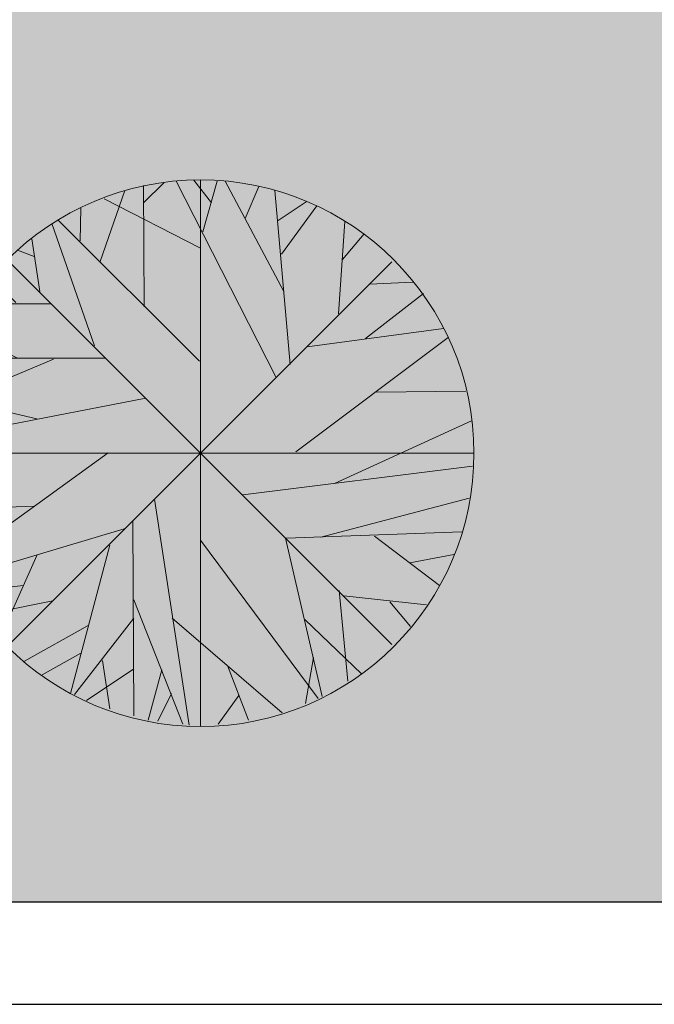
# Model space of a CAD drawing. Units: inches. Extents: x 459864 to 460310, y 324185 to 324787.
# Tile 72 of 112: x 460210 to 460238, y 324195 to 324238. Entities that reach past the tile are written whole.
import ezdxf

# ---------------------------------------------------------------- set-up
doc = ezdxf.new("R2010")
doc.units = ezdxf.units.IN
for name, color, linetype, lineweight in [('C-PROP', 7, 'Continuous', 30), ('L-PLNT', 3, 'Continuous', 13), ('L-SITE-PATT', 252, 'Continuous', 13)]:
    doc.layers.add(name, color=color, linetype=linetype, lineweight=lineweight)

# ---------------------------------------------------------------- blocks, each defined once
blk = doc.blocks.new('Tree - deciduous plan')
for p, q in [((-12.5388, 54.9406), (-7.9613, 59.4546)), ((-12.3627, 32.1443), (-12.5388, 58.7776)), ((-5.3205, 59.6806), (16.5105, 16.7963)), ((2.426, 54.9406), (-1.4472, 59.9056)), ((0, 59.9996), (0, -60)), ((0.4894, 48.6208), (3.6584, 59.6806)), ((18.2711, 35.5298), (5.419, 59.6806)), ((9.8203, 51.5549), (12.8133, 58.5516)), ((-22.0458, 42.0753), (-16.5881, 57.6486)), ((19.6795, 19.5047), (16.3344, 57.6486)), ((-21.1656, 55.8436), (-0.0388, 45.0094)), ((17.0387, 51.1035), (23.2006, 55.1666)), ((17.7429, 43.6552), (25.4894, 54.2636)), ((-26.4472, 46.5894), (-26.2712, 53.8116)), ((-32.6092, 50.4264), (-23.2782, 23.5674)), ((-31.2008, 51.1035), (-0.2149, 20.1818)), ((31.6513, 50.8778), (30.2429, 30.5643)), ((31.1232, 42.5267), (35.8767, 48.1693)), ((-37.0107, 47.0408), (-35.25, 35.5298)), ((-40.1797, 44.558), (-36.4825, 43.2038)), ((42, 42), (-42, -42)), ((42, -42), (-42, 42)), ((-43.8768, 36.4326), (-44.405, 40.2696)), ((-45.8134, 38.2383), (-40.5318, 33.0471)), ((37.1091, 37.1098), (46.6161, 37.5612)), ((36.2288, 25.1474), (48.9049, 35.0784)), ((-49.8627, 32.8214), (-32.7853, 32.8214)), ((-53.2078, 27.4044), (-40.1797, 20.859)), ((23.3767, 23.3417), (53.3063, 27.4044)), ((-54.7923, 24.4702), (-47.75, 21.0847)), ((54.3626, 25.3731), (20.9119, 0.3198)), ((-32.2571, 20.6333), (-59.1937, 9.348)), ((-56.0247, 20.859), (-20.8134, 20.859)), ((-57.081, 17.9248), (-47.0458, 14.7649)), ((38.5175, 13.4107), (58.2359, 13.6364)), ((-59.7219, 2.8025), (-12.0106, 12.0565)), ((-58.6656, 12.7336), (-35.9543, 7.5424)), ((29.3626, -6.6771), (59.4682, 7.091)), ((-54.6162, -24.7335), (-20.2853, 0.0941)), ((-60, 0), (60, 0)), ((-45.2853, -0.1316), (-59.0177, -10.0627)), ((9.2922, -9.1598), (59.6443, -2.8401)), ((-59.7219, -4.8714), (-54.2641, -6.6771)), ((-10.074, -10.0627), (-2.5036, -59.7178)), ((26.3697, -18.4138), (58.9401, -9.8369)), ((-58.4895, -12.3197), (-36.4825, -11.6426)), ((-14.8275, -15.0282), (-14.6515, -57.6865)), ((-53.2078, -27.442), (-16.7641, -16.6081)), ((18.7992, -18.6394), (57.3556, -17.2853)), ((-57.081, -18.4138), (-45.2853, -17.9624)), ((-52.6797, -18.188), (-55.4966, -22.0251)), ((-47.2219, -19.3166), (-50.2148, -26.3135)), ((-0.0388, -19.0909), (25.8415, -53.8495)), ((18.6232, -18.6394), (26.7218, -53.3981)), ((38.1654, -18.188), (52.426, -29.0219)), ((-19.9331, -20.2194), (-28.5599, -52.721)), ((-35.9543, -22.4765), (-44.0529, -40.5329)), ((45.9119, -24.0564), (55.595, -22.2508)), ((-38.9472, -29.0219), (-51.4472, -30.6018)), ((-46.5177, -30.1504), (-49.5106, -33.536)), ((30.419, -30.1504), (32.3556, -50.0125)), ((-32.4331, -32.4075), (-48.1021, -35.5674)), ((-14.6515, -32.1818), (-3.912, -59.4922)), ((31.4753, -31.279), (49.6091, -33.3103)), ((41.5105, -32.6332), (46.088, -38.0501)), ((-43.7008, -34.6645), (-46.6937, -37.373)), ((-14.6515, -36.2445), (-27.6797, -52.9467)), ((-6.2008, -36.2445), (17.919, -57.0094)), ((22.8485, -36.4702), (35.3485, -48.4326)), ((-24.6867, -37.8244), (-38.7712, -45.7241)), ((-26.2712, -43.9185), (-34.7219, -48.6583)), ((24.7852, -44.8213), (23.0246, -54.978)), ((-14.6515, -47.3041), (-25.0388, -54.3009)), ((-21.5177, -45.4984), (-19.9331, -56.1065)), ((-8.4895, -47.5298), (-11.4825, -58.5893)), ((5.9471, -46.6269), (10.5246, -58.5893)), ((-6.3768, -52.721), (-9.3698, -58.815)), ((8.4119, -53.1724), (3.8344, -59.4922))]:
    blk.add_line(p, q)
blk.add_circle((0, 0), 60)

msp = doc.modelspace()

# ---------------------------------------------------------------- hatches: boundary and pattern name
at = {"layer": 'L-SITE-PATT'}
h = msp.add_hatch(dxfattribs=at)
h.set_pattern_fill('DOTS', color=256)
h.paths.add_polyline_path([(460269.804, 324283.483), (460247.115, 324283.483), (460121.929, 324283.483), (460121.929, 324252.473), (460117.429, 324252.473), (460110.124, 324252.473), (460110.124, 324243.287), (460080.83, 324243.287), (460080.83, 324252.473), (460061.115, 324252.473), (460061.115, 324251.882), (460077.909, 324251.882), (460077.909, 324199.483), (460080.83, 324199.483), (460080.83, 324207.553), (460110.124, 324207.553), (460110.124, 324199.483), (460110.813, 324199.483), (460262.115, 324199.483), (460269.804, 324199.483)], flags=17)
edge = h.paths.add_edge_path(flags=0)
edge.add_ellipse((460222.59, 324263.813), major_axis=(-8.485, 8.485), ratio=1, start_angle=405, end_angle=495, ccw=False)
edge.add_line((460214.821, 324254.66), (460214.832, 324254.666))
edge.add_ellipse((460222.59, 324263.813), major_axis=(-8.485, 8.485), ratio=1, start_angle=405, end_angle=495, ccw=False)
edge.add_line((460210.759, 324261.781), (460210.768, 324261.787))
edge.add_ellipse((460222.59, 324263.813), major_axis=(-8.485, 8.485), ratio=1, start_angle=405, end_angle=495, ccw=False)
edge.add_ellipse((460222.59, 324263.813), major_axis=(-8.485, 8.485), ratio=1, start_angle=392.754, end_angle=405, ccw=False)
edge.add_ellipse((460222.59, 324263.813), major_axis=(-8.485, 8.485), ratio=1, start_angle=380.9347, end_angle=392.754, ccw=False)
edge.add_line((460211.337, 324267.985), (460211.34, 324267.985))
edge.add_ellipse((460222.59, 324263.813), major_axis=(-8.485, 8.485), ratio=1, start_angle=380.9347, end_angle=392.754, ccw=False)
edge.add_ellipse((460222.59, 324263.813), major_axis=(-8.485, 8.485), ratio=1, start_angle=347.9015, end_angle=380.9347, ccw=False)
edge.add_ellipse((460222.59, 324263.813), major_axis=(-8.485, 8.485), ratio=1, start_angle=327.0619, end_angle=347.9015, ccw=False)
edge.add_ellipse((460222.59, 324263.813), major_axis=(-8.485, 8.485), ratio=1, start_angle=278.3246, end_angle=327.0619, ccw=False)
edge.add_line((460225.158, 324275.536), (460225.158, 324275.535))
edge.add_ellipse((460222.59, 324263.813), major_axis=(-8.485, 8.485), ratio=1, start_angle=278.3246, end_angle=327.0619, ccw=False)
edge.add_ellipse((460222.59, 324263.813), major_axis=(-8.485, 8.485), ratio=1, start_angle=260.6436, end_angle=278.3246, ccw=False)
edge.add_ellipse((460222.59, 324263.813), major_axis=(-8.485, 8.485), ratio=1, start_angle=225, end_angle=260.6436, ccw=False)
edge.add_line((460234.509, 324265.243), (460234.501, 324265.239))
edge.add_ellipse((460222.59, 324263.813), major_axis=(-8.485, 8.485), ratio=1, start_angle=225, end_angle=260.6436, ccw=False)
edge.add_ellipse((460222.59, 324263.813), major_axis=(-8.485, 8.485), ratio=1, start_angle=495, end_angle=585, ccw=False)
edge.add_line((460234.437, 324261.861), (460234.424, 324261.858))
edge.add_ellipse((460222.59, 324263.813), major_axis=(-8.485, 8.485), ratio=1, start_angle=495, end_angle=585, ccw=False)
edge.add_line((460227.95, 324253.067), (460227.946, 324253.083))
edge.add_ellipse((460222.59, 324263.813), major_axis=(-8.485, 8.485), ratio=1, start_angle=495, end_angle=585, ccw=False)
edge.add_line((460226.223, 324252.369), (460226.211, 324252.38))
edge.add_ellipse((460222.59, 324263.813), major_axis=(-8.485, 8.485), ratio=1, start_angle=495, end_angle=585, ccw=False)
h.paths.add_polyline_path([(460219.651, 324254.347), (460218.461, 324253.545), (460218.275, 324254.789), (460219.642, 324256.542), (460219.625, 324260.848), (460216.11, 324257.333), (460214.35, 324256.978), (460215.416, 324259.356), (460212.524, 324258.496), (460213.137, 324259.93), (460218.507, 324263.813), (460222.59, 324263.813), (460222.59, 324267.807), (460218.176, 324272.212), (460219.026, 324274.639), (460222.59, 324272.811), (460222.59, 324275.423), (460223.057, 324274.825), (460222.675, 324273.492), (460225.912, 324267.135), (460219.625, 324260.848)], flags=0)
edge = h.paths.add_edge_path(flags=0)
edge.add_ellipse((460194.576, 324264.046), major_axis=(-8.485, 8.485), ratio=1, start_angle=495, end_angle=585, ccw=False)
edge.add_line((460199.936, 324253.3), (460199.932, 324253.316))
edge.add_ellipse((460194.576, 324264.046), major_axis=(-8.485, 8.485), ratio=1, start_angle=495, end_angle=585, ccw=False)
edge.add_line((460198.208, 324252.603), (460198.196, 324252.613))
edge.add_ellipse((460194.576, 324264.046), major_axis=(-8.485, 8.485), ratio=1, start_angle=495, end_angle=585, ccw=False)
edge.add_ellipse((460194.576, 324264.046), major_axis=(-8.485, 8.485), ratio=1, start_angle=405, end_angle=495, ccw=False)
edge.add_line((460186.806, 324254.893), (460186.817, 324254.899))
edge.add_ellipse((460194.576, 324264.046), major_axis=(-8.485, 8.485), ratio=1, start_angle=405, end_angle=495, ccw=False)
edge.add_line((460182.744, 324262.014), (460182.753, 324262.02))
edge.add_ellipse((460194.576, 324264.046), major_axis=(-8.485, 8.485), ratio=1, start_angle=405, end_angle=495, ccw=False)
edge.add_ellipse((460194.576, 324264.046), major_axis=(-8.485, 8.485), ratio=1, start_angle=392.754, end_angle=405, ccw=False)
edge.add_ellipse((460194.576, 324264.046), major_axis=(-8.485, 8.485), ratio=1, start_angle=380.9347, end_angle=392.754, ccw=False)
edge.add_line((460183.323, 324268.218), (460183.326, 324268.218))
edge.add_ellipse((460194.576, 324264.046), major_axis=(-8.485, 8.485), ratio=1, start_angle=380.9347, end_angle=392.754, ccw=False)
edge.add_ellipse((460194.576, 324264.046), major_axis=(-8.485, 8.485), ratio=1, start_angle=347.9015, end_angle=380.9347, ccw=False)
edge.add_ellipse((460194.576, 324264.046), major_axis=(-8.485, 8.485), ratio=1, start_angle=327.0619, end_angle=347.9015, ccw=False)
edge.add_ellipse((460194.576, 324264.046), major_axis=(-8.485, 8.485), ratio=1, start_angle=278.3246, end_angle=327.0619, ccw=False)
edge.add_line((460197.144, 324275.769), (460197.143, 324275.768))
edge.add_ellipse((460194.576, 324264.046), major_axis=(-8.485, 8.485), ratio=1, start_angle=278.3246, end_angle=327.0619, ccw=False)
edge.add_ellipse((460194.576, 324264.046), major_axis=(-8.485, 8.485), ratio=1, start_angle=260.6436, end_angle=278.3246, ccw=False)
edge.add_ellipse((460194.576, 324264.046), major_axis=(-8.485, 8.485), ratio=1, start_angle=225, end_angle=260.6436, ccw=False)
edge.add_line((460206.494, 324265.476), (460206.487, 324265.473))
edge.add_ellipse((460194.576, 324264.046), major_axis=(-8.485, 8.485), ratio=1, start_angle=225, end_angle=260.6436, ccw=False)
edge.add_ellipse((460194.576, 324264.046), major_axis=(-8.485, 8.485), ratio=1, start_angle=495, end_angle=585, ccw=False)
edge.add_line((460206.422, 324262.094), (460206.409, 324262.091))
h.paths.add_polyline_path([(460191.61, 324261.081), (460191.637, 324254.58), (460190.447, 324253.778), (460190.261, 324255.023), (460191.628, 324256.775), (460191.61, 324261.081), (460188.096, 324257.566), (460186.335, 324257.211), (460187.402, 324259.589), (460184.509, 324258.729), (460185.123, 324260.163), (460190.493, 324264.046), (460194.576, 324264.046), (460194.576, 324268.04), (460190.161, 324272.446), (460191.011, 324274.872), (460194.576, 324273.044), (460194.576, 324275.657), (460195.043, 324275.058), (460194.661, 324273.725), (460197.897, 324267.368)], flags=0)
edge = h.paths.add_edge_path(flags=0)
edge.add_ellipse((460252.912, 324263.578), major_axis=(-8.485, 8.485), ratio=1, start_angle=405, end_angle=495, ccw=False)
edge.add_line((460241.081, 324261.545), (460241.089, 324261.551))
edge.add_ellipse((460252.912, 324263.578), major_axis=(-8.485, 8.485), ratio=1, start_angle=405, end_angle=495, ccw=False)
edge.add_ellipse((460252.912, 324263.578), major_axis=(-8.485, 8.485), ratio=1, start_angle=392.754, end_angle=405, ccw=False)
edge.add_ellipse((460252.912, 324263.578), major_axis=(-8.485, 8.485), ratio=1, start_angle=380.9347, end_angle=392.754, ccw=False)
edge.add_line((460241.659, 324267.749), (460241.662, 324267.749))
edge.add_ellipse((460252.912, 324263.578), major_axis=(-8.485, 8.485), ratio=1, start_angle=380.9347, end_angle=392.754, ccw=False)
edge.add_ellipse((460252.912, 324263.578), major_axis=(-8.485, 8.485), ratio=1, start_angle=347.9015, end_angle=380.9347, ccw=False)
edge.add_ellipse((460252.912, 324263.578), major_axis=(-8.485, 8.485), ratio=1, start_angle=327.0619, end_angle=347.9015, ccw=False)
edge.add_ellipse((460252.912, 324263.578), major_axis=(-8.485, 8.485), ratio=1, start_angle=278.3246, end_angle=327.0619, ccw=False)
edge.add_line((460255.48, 324275.3), (460255.479, 324275.299))
edge.add_ellipse((460252.912, 324263.578), major_axis=(-8.485, 8.485), ratio=1, start_angle=278.3246, end_angle=327.0619, ccw=False)
edge.add_ellipse((460252.912, 324263.578), major_axis=(-8.485, 8.485), ratio=1, start_angle=260.6436, end_angle=278.3246, ccw=False)
edge.add_ellipse((460252.912, 324263.578), major_axis=(-8.485, 8.485), ratio=1, start_angle=225, end_angle=260.6436, ccw=False)
edge.add_line((460264.83, 324265.007), (460264.823, 324265.004))
edge.add_ellipse((460252.912, 324263.578), major_axis=(-8.485, 8.485), ratio=1, start_angle=225, end_angle=260.6436, ccw=False)
edge.add_ellipse((460252.912, 324263.578), major_axis=(-8.485, 8.485), ratio=1, start_angle=495, end_angle=585, ccw=False)
edge.add_line((460264.758, 324261.626), (460264.745, 324261.622))
edge.add_ellipse((460252.912, 324263.578), major_axis=(-8.485, 8.485), ratio=1, start_angle=495, end_angle=585, ccw=False)
edge.add_line((460258.272, 324252.832), (460258.268, 324252.848))
edge.add_ellipse((460252.912, 324263.578), major_axis=(-8.485, 8.485), ratio=1, start_angle=495, end_angle=585, ccw=False)
edge.add_line((460256.545, 324252.134), (460256.533, 324252.144))
edge.add_ellipse((460252.912, 324263.578), major_axis=(-8.485, 8.485), ratio=1, start_angle=495, end_angle=585, ccw=False)
edge.add_ellipse((460252.912, 324263.578), major_axis=(-8.485, 8.485), ratio=1, start_angle=405, end_angle=495, ccw=False)
edge.add_line((460245.143, 324254.424), (460245.153, 324254.43))
h.paths.add_polyline_path([(460244.672, 324256.742), (460245.738, 324259.12), (460242.846, 324258.26), (460243.459, 324259.694), (460248.829, 324263.578), (460252.912, 324263.578), (460252.912, 324267.571), (460248.497, 324271.977), (460249.348, 324274.403), (460252.912, 324272.576), (460252.912, 324275.188), (460253.379, 324274.589), (460252.997, 324273.257), (460256.233, 324266.899), (460249.946, 324260.612), (460249.973, 324254.111), (460248.783, 324253.309), (460248.597, 324254.554), (460249.964, 324256.306), (460249.946, 324260.612), (460246.432, 324257.097)], flags=0)
edge = h.paths.add_edge_path(flags=0)
edge.add_ellipse((460167.439, 324262.833), major_axis=(-8.485, 8.485), ratio=1, start_angle=495, end_angle=585, ccw=False)
edge.add_line((460172.799, 324252.087), (460172.795, 324252.103))
edge.add_ellipse((460167.439, 324262.833), major_axis=(-8.485, 8.485), ratio=1, start_angle=495, end_angle=585, ccw=False)
edge.add_line((460171.071, 324251.389), (460171.059, 324251.399))
edge.add_ellipse((460167.439, 324262.833), major_axis=(-8.485, 8.485), ratio=1, start_angle=495, end_angle=585, ccw=False)
edge.add_ellipse((460167.439, 324262.833), major_axis=(-8.485, 8.485), ratio=1, start_angle=405, end_angle=495, ccw=False)
edge.add_line((460159.669, 324253.679), (460159.68, 324253.685))
edge.add_ellipse((460167.439, 324262.833), major_axis=(-8.485, 8.485), ratio=1, start_angle=405, end_angle=495, ccw=False)
edge.add_line((460155.607, 324260.8), (460155.616, 324260.806))
edge.add_ellipse((460167.439, 324262.833), major_axis=(-8.485, 8.485), ratio=1, start_angle=405, end_angle=495, ccw=False)
edge.add_ellipse((460167.439, 324262.833), major_axis=(-8.485, 8.485), ratio=1, start_angle=392.754, end_angle=405, ccw=False)
edge.add_ellipse((460167.439, 324262.833), major_axis=(-8.485, 8.485), ratio=1, start_angle=380.9347, end_angle=392.754, ccw=False)
edge.add_line((460156.185, 324267.005), (460156.189, 324267.005))
edge.add_ellipse((460167.439, 324262.833), major_axis=(-8.485, 8.485), ratio=1, start_angle=380.9347, end_angle=392.754, ccw=False)
edge.add_ellipse((460167.439, 324262.833), major_axis=(-8.485, 8.485), ratio=1, start_angle=347.9015, end_angle=380.9347, ccw=False)
edge.add_ellipse((460167.439, 324262.833), major_axis=(-8.485, 8.485), ratio=1, start_angle=327.0619, end_angle=347.9015, ccw=False)
edge.add_ellipse((460167.439, 324262.833), major_axis=(-8.485, 8.485), ratio=1, start_angle=278.3246, end_angle=327.0619, ccw=False)
edge.add_line((460170.007, 324274.556), (460170.006, 324274.554))
edge.add_ellipse((460167.439, 324262.833), major_axis=(-8.485, 8.485), ratio=1, start_angle=278.3246, end_angle=327.0619, ccw=False)
edge.add_ellipse((460167.439, 324262.833), major_axis=(-8.485, 8.485), ratio=1, start_angle=260.6436, end_angle=278.3246, ccw=False)
edge.add_ellipse((460167.439, 324262.833), major_axis=(-8.485, 8.485), ratio=1, start_angle=225, end_angle=260.6436, ccw=False)
edge.add_line((460179.357, 324264.262), (460179.35, 324264.259))
edge.add_ellipse((460167.439, 324262.833), major_axis=(-8.485, 8.485), ratio=1, start_angle=225, end_angle=260.6436, ccw=False)
edge.add_ellipse((460167.439, 324262.833), major_axis=(-8.485, 8.485), ratio=1, start_angle=495, end_angle=585, ccw=False)
edge.add_line((460179.285, 324260.881), (460179.272, 324260.877))
h.paths.add_polyline_path([(460164.473, 324259.867), (460164.5, 324253.366), (460163.31, 324252.565), (460163.124, 324253.809), (460164.491, 324255.561), (460164.473, 324259.867), (460160.958, 324256.353), (460159.198, 324255.998), (460160.265, 324258.375), (460157.372, 324257.515), (460157.986, 324258.949), (460163.356, 324262.833), (460167.439, 324262.833), (460167.439, 324266.826), (460163.024, 324271.232), (460163.874, 324273.659), (460167.439, 324271.831), (460167.439, 324274.443), (460167.905, 324273.844), (460167.524, 324272.512), (460170.76, 324266.154)], flags=0)
edge = h.paths.add_edge_path(flags=0)
edge.add_ellipse((460140.758, 324262.37), major_axis=(-8.485, 8.485), ratio=1, start_angle=495, end_angle=585, ccw=False)
edge.add_line((460146.118, 324251.624), (460146.114, 324251.639))
edge.add_ellipse((460140.758, 324262.37), major_axis=(-8.485, 8.485), ratio=1, start_angle=495, end_angle=585, ccw=False)
edge.add_line((460144.391, 324250.926), (460144.379, 324250.936))
edge.add_ellipse((460140.758, 324262.37), major_axis=(-8.485, 8.485), ratio=1, start_angle=495, end_angle=585, ccw=False)
edge.add_ellipse((460140.758, 324262.37), major_axis=(-8.485, 8.485), ratio=1, start_angle=405, end_angle=495, ccw=False)
edge.add_line((460132.989, 324253.216), (460132.999, 324253.222))
edge.add_ellipse((460140.758, 324262.37), major_axis=(-8.485, 8.485), ratio=1, start_angle=405, end_angle=495, ccw=False)
edge.add_line((460128.927, 324260.337), (460128.935, 324260.343))
edge.add_ellipse((460140.758, 324262.37), major_axis=(-8.485, 8.485), ratio=1, start_angle=405, end_angle=495, ccw=False)
edge.add_ellipse((460140.758, 324262.37), major_axis=(-8.485, 8.485), ratio=1, start_angle=392.754, end_angle=405, ccw=False)
edge.add_ellipse((460140.758, 324262.37), major_axis=(-8.485, 8.485), ratio=1, start_angle=380.9347, end_angle=392.754, ccw=False)
edge.add_line((460129.505, 324266.541), (460129.508, 324266.541))
edge.add_ellipse((460140.758, 324262.37), major_axis=(-8.485, 8.485), ratio=1, start_angle=380.9347, end_angle=392.754, ccw=False)
edge.add_ellipse((460140.758, 324262.37), major_axis=(-8.485, 8.485), ratio=1, start_angle=347.9015, end_angle=380.9347, ccw=False)
edge.add_ellipse((460140.758, 324262.37), major_axis=(-8.485, 8.485), ratio=1, start_angle=327.0619, end_angle=347.9015, ccw=False)
edge.add_ellipse((460140.758, 324262.37), major_axis=(-8.485, 8.485), ratio=1, start_angle=278.3246, end_angle=327.0619, ccw=False)
edge.add_line((460143.326, 324274.092), (460143.325, 324274.091))
edge.add_ellipse((460140.758, 324262.37), major_axis=(-8.485, 8.485), ratio=1, start_angle=278.3246, end_angle=327.0619, ccw=False)
edge.add_ellipse((460140.758, 324262.37), major_axis=(-8.485, 8.485), ratio=1, start_angle=260.6436, end_angle=278.3246, ccw=False)
edge.add_ellipse((460140.758, 324262.37), major_axis=(-8.485, 8.485), ratio=1, start_angle=225, end_angle=260.6436, ccw=False)
edge.add_line((460152.677, 324263.799), (460152.669, 324263.796))
edge.add_ellipse((460140.758, 324262.37), major_axis=(-8.485, 8.485), ratio=1, start_angle=225, end_angle=260.6436, ccw=False)
edge.add_ellipse((460140.758, 324262.37), major_axis=(-8.485, 8.485), ratio=1, start_angle=495, end_angle=585, ccw=False)
edge.add_line((460152.604, 324260.418), (460152.592, 324260.414))
h.paths.add_polyline_path([(460137.792, 324259.404), (460137.819, 324252.903), (460136.629, 324252.101), (460136.443, 324253.346), (460137.81, 324255.098), (460137.792, 324259.404), (460134.278, 324255.889), (460132.518, 324255.534), (460133.584, 324257.912), (460130.692, 324257.052), (460131.305, 324258.486), (460136.675, 324262.37), (460140.758, 324262.37), (460140.758, 324266.363), (460136.343, 324270.769), (460137.194, 324273.195), (460140.758, 324271.367), (460140.758, 324273.98), (460141.225, 324273.381), (460140.843, 324272.049), (460144.079, 324265.691)], flags=0)
h.paths.add_polyline_path([(460110.124, 324227.414), (460080.83, 324227.414), (460080.83, 324235.484), (460110.124, 324235.484)], flags=16)
h.paths.add_polyline_path([(460110.124, 324220.797), (460110.124, 324212.727), (460080.83, 324212.727), (460080.83, 324220.797)], flags=16)
h.paths.add_polyline_path([(460269.804, 324283.483), (460247.115, 324283.483), (460121.929, 324283.483), (460121.929, 324252.473), (460117.429, 324252.473), (460110.124, 324252.473), (460110.124, 324243.287), (460080.83, 324243.287), (460080.83, 324252.473), (460061.115, 324252.473), (460061.115, 324251.882), (460077.909, 324251.882), (460077.909, 324199.483), (460080.83, 324199.483), (460080.83, 324207.553), (460110.124, 324207.553), (460110.124, 324199.483), (460262.115, 324199.483), (460269.804, 324199.483)], flags=17)
h.paths.add_polyline_path([(460219.651, 324254.347), (460218.461, 324253.545), (460218.275, 324254.789), (460219.642, 324256.542), (460219.625, 324260.848), (460216.11, 324257.333), (460214.35, 324256.978), (460215.416, 324259.356), (460212.524, 324258.496), (460213.137, 324259.93), (460218.507, 324263.813), (460222.59, 324263.813), (460220.18, 324266.223), (460215.461, 324265.308), (460211.835, 324266.137), (460216.247, 324267.985), (460218.418, 324267.985), (460222.59, 324263.813), (460222.59, 324267.807), (460218.176, 324272.212), (460219.026, 324274.639), (460222.59, 324272.811), (460222.59, 324275.423), (460223.057, 324274.825), (460222.675, 324273.492), (460225.912, 324267.135), (460222.59, 324263.813), (460231.383, 324263.813), (460228.485, 324262.488), (460224.425, 324261.978), (460228.68, 324257.724), (460228.966, 324254.791), (460227.142, 324256.537), (460227.542, 324254.819), (460227.333, 324253.614), (460222.59, 324259.985), (460222.59, 324255.497), (460221.377, 324256.541), (460220.576, 324261.799), (460219.625, 324260.848)], flags=0)
h.paths.add_polyline_path([(460199.127, 324256.77), (460199.528, 324255.052), (460199.319, 324253.848), (460194.576, 324260.218), (460194.576, 324255.73), (460193.363, 324256.774), (460192.561, 324262.032), (460191.61, 324261.081), (460191.637, 324254.58), (460190.447, 324253.778), (460190.261, 324255.023), (460191.628, 324256.775), (460191.61, 324261.081), (460188.096, 324257.566), (460186.335, 324257.211), (460187.402, 324259.589), (460184.509, 324258.729), (460185.123, 324260.163), (460190.493, 324264.046), (460194.576, 324264.046), (460192.166, 324266.456), (460187.446, 324265.541), (460183.82, 324266.37), (460188.232, 324268.218), (460190.404, 324268.218), (460194.576, 324264.046), (460194.576, 324268.04), (460190.161, 324272.446), (460191.011, 324274.872), (460194.576, 324273.044), (460194.576, 324275.657), (460195.043, 324275.058), (460194.661, 324273.725), (460197.897, 324267.368), (460194.576, 324264.046), (460203.368, 324264.046), (460200.47, 324262.721), (460196.411, 324262.212), (460200.665, 324257.957), (460200.951, 324255.024)], flags=0)
h.paths.add_polyline_path([(460244.672, 324256.742), (460245.738, 324259.12), (460242.846, 324258.26), (460243.459, 324259.694), (460248.829, 324263.578), (460252.912, 324263.578), (460250.502, 324265.987), (460245.783, 324265.072), (460242.156, 324265.901), (460246.568, 324267.749), (460248.74, 324267.749), (460252.912, 324263.578), (460252.912, 324267.571), (460248.497, 324271.977), (460249.348, 324274.403), (460252.912, 324272.576), (460252.912, 324275.188), (460253.379, 324274.589), (460252.997, 324273.257), (460256.233, 324266.899), (460252.912, 324263.578), (460261.705, 324263.578), (460258.806, 324262.252), (460254.747, 324261.743), (460259.002, 324257.488), (460259.288, 324254.555), (460257.463, 324256.301), (460257.864, 324254.583), (460257.655, 324253.379), (460252.912, 324259.749), (460252.912, 324255.261), (460251.699, 324256.305), (460250.897, 324261.563), (460249.946, 324260.612), (460249.973, 324254.111), (460248.783, 324253.309), (460248.597, 324254.554), (460249.964, 324256.306), (460249.946, 324260.612), (460246.432, 324257.097)], flags=0)
h.paths.add_polyline_path([(460173.528, 324256.743), (460173.814, 324253.811), (460171.99, 324255.556), (460172.39, 324253.838), (460172.182, 324252.634), (460167.439, 324259.004), (460167.439, 324254.516), (460166.226, 324255.56), (460165.424, 324260.818), (460164.473, 324259.867), (460164.5, 324253.366), (460163.31, 324252.565), (460163.124, 324253.809), (460164.491, 324255.561), (460164.473, 324259.867), (460160.958, 324256.353), (460159.198, 324255.998), (460160.265, 324258.375), (460157.372, 324257.515), (460157.986, 324258.949), (460163.356, 324262.833), (460167.439, 324262.833), (460165.029, 324265.243), (460160.309, 324264.327), (460156.683, 324265.156), (460161.095, 324267.005), (460163.267, 324267.005), (460167.439, 324262.833), (460167.439, 324266.826), (460163.024, 324271.232), (460163.874, 324273.659), (460167.439, 324271.831), (460167.439, 324274.443), (460167.905, 324273.844), (460167.524, 324272.512), (460170.76, 324266.154), (460167.439, 324262.833), (460176.231, 324262.833), (460173.333, 324261.507), (460169.274, 324260.998)], flags=0)
h.paths.add_polyline_path([(460146.848, 324256.28), (460147.134, 324253.347), (460145.31, 324255.093), (460145.71, 324253.375), (460145.501, 324252.171), (460140.758, 324258.541), (460140.758, 324254.053), (460139.545, 324255.097), (460138.744, 324260.355), (460137.792, 324259.404), (460137.819, 324252.903), (460136.629, 324252.101), (460136.443, 324253.346), (460137.81, 324255.098), (460137.792, 324259.404), (460134.278, 324255.889), (460132.518, 324255.534), (460133.584, 324257.912), (460130.692, 324257.052), (460131.305, 324258.486), (460136.675, 324262.37), (460140.758, 324262.37), (460138.348, 324264.779), (460133.629, 324263.864), (460130.002, 324264.693), (460134.414, 324266.541), (460136.586, 324266.541), (460140.758, 324262.37), (460140.758, 324266.363), (460136.343, 324270.769), (460137.194, 324273.195), (460140.758, 324271.367), (460140.758, 324273.98), (460141.225, 324273.381), (460140.843, 324272.049), (460144.079, 324265.691), (460140.758, 324262.37), (460149.551, 324262.37), (460146.653, 324261.044), (460142.593, 324260.535)], flags=0)
edge = h.paths.add_edge_path()
edge.add_line((460269.804, 324272.549), (460260.881, 324272.549))
edge.add_ellipse((460252.912, 324263.578), major_axis=(-8.485, 8.485), ratio=1, start_angle=260.6436, end_angle=273.3846, ccw=False)
edge.add_line((460262.283, 324271.092), (460262.261, 324271.091))
edge.add_ellipse((460252.912, 324263.578), major_axis=(-8.485, 8.485), ratio=1, start_angle=260.6436, end_angle=273.3846, ccw=False)
edge.add_ellipse((460252.912, 324263.578), major_axis=(-8.485, 8.485), ratio=1, start_angle=225, end_angle=260.6436, ccw=False)
edge.add_line((460263.609, 324269.063), (460263.572, 324269.058))
edge.add_ellipse((460252.912, 324263.578), major_axis=(-8.485, 8.485), ratio=1, start_angle=225, end_angle=260.6436, ccw=False)
edge.add_line((460264.615, 324266.306), (460264.585, 324266.305))
edge.add_ellipse((460252.912, 324263.578), major_axis=(-8.485, 8.485), ratio=1, start_angle=225, end_angle=260.6436, ccw=False)
edge.add_line((460264.83, 324265.007), (460264.823, 324265.004))
edge.add_ellipse((460252.912, 324263.578), major_axis=(-8.485, 8.485), ratio=1, start_angle=225, end_angle=260.6436, ccw=False)
edge.add_ellipse((460252.912, 324263.578), major_axis=(-8.485, 8.485), ratio=1, start_angle=495, end_angle=585, ccw=False)
edge.add_line((460264.758, 324261.626), (460264.745, 324261.622))
edge.add_ellipse((460252.912, 324263.578), major_axis=(-8.485, 8.485), ratio=1, start_angle=495, end_angle=585, ccw=False)
edge.add_line((460263.442, 324257.739), (460263.389, 324257.779))
edge.add_ellipse((460252.912, 324263.578), major_axis=(-8.485, 8.485), ratio=1, start_angle=495, end_angle=585, ccw=False)
edge.add_line((460258.128, 324252.744), (460258.102, 324252.779))
edge.add_ellipse((460252.912, 324263.578), major_axis=(-8.485, 8.485), ratio=1, start_angle=495, end_angle=585, ccw=False)
edge.add_line((460256.545, 324252.134), (460256.533, 324252.144))
edge.add_ellipse((460252.912, 324263.578), major_axis=(-8.485, 8.485), ratio=1, start_angle=495, end_angle=585, ccw=False)
edge.add_ellipse((460252.912, 324263.578), major_axis=(-8.485, 8.485), ratio=1, start_angle=405, end_angle=495, ccw=False)
edge.add_line((460250.594, 324251.78), (460250.605, 324251.82))
edge.add_ellipse((460252.912, 324263.578), major_axis=(-8.485, 8.485), ratio=1, start_angle=405, end_angle=495, ccw=False)
edge.add_line((460245.143, 324254.424), (460245.153, 324254.43))
edge.add_ellipse((460252.912, 324263.578), major_axis=(-8.485, 8.485), ratio=1, start_angle=405, end_angle=495, ccw=False)
edge.add_line((460243.525, 324256.059), (460243.56, 324256.091))
edge.add_ellipse((460252.912, 324263.578), major_axis=(-8.485, 8.485), ratio=1, start_angle=405, end_angle=495, ccw=False)
edge.add_line((460241.44, 324259.893), (460241.522, 324259.896))
edge.add_ellipse((460252.912, 324263.578), major_axis=(-8.485, 8.485), ratio=1, start_angle=405, end_angle=495, ccw=False)
edge.add_line((460241.081, 324261.545), (460241.089, 324261.551))
edge.add_ellipse((460252.912, 324263.578), major_axis=(-8.485, 8.485), ratio=1, start_angle=405, end_angle=495, ccw=False)
edge.add_ellipse((460252.912, 324263.578), major_axis=(-8.485, 8.485), ratio=1, start_angle=392.754, end_angle=405, ccw=False)
edge.add_line((460241.05, 324265.438), (460241.063, 324265.443))
edge.add_ellipse((460252.912, 324263.578), major_axis=(-8.485, 8.485), ratio=1, start_angle=392.754, end_angle=405, ccw=False)
edge.add_ellipse((460252.912, 324263.578), major_axis=(-8.485, 8.485), ratio=1, start_angle=380.9347, end_angle=392.754, ccw=False)
edge.add_line((460241.452, 324267.176), (460241.469, 324267.171))
edge.add_ellipse((460252.912, 324263.578), major_axis=(-8.485, 8.485), ratio=1, start_angle=380.9347, end_angle=392.754, ccw=False)
edge.add_line((460241.659, 324267.749), (460241.662, 324267.749))
edge.add_ellipse((460252.912, 324263.578), major_axis=(-8.485, 8.485), ratio=1, start_angle=380.9347, end_angle=392.754, ccw=False)
edge.add_ellipse((460252.912, 324263.578), major_axis=(-8.485, 8.485), ratio=1, start_angle=356.6154, end_angle=380.9347, ccw=False)
edge.add_line((460244.88, 324272.488), (460244.713, 324272.549))
edge.add_line((460244.713, 324272.549), (460230.817, 324272.549))
edge.add_ellipse((460222.59, 324263.813), major_axis=(-8.485, 8.485), ratio=1, start_angle=260.6436, end_angle=271.7178, ccw=False)
edge.add_ellipse((460222.59, 324263.813), major_axis=(-8.485, 8.485), ratio=1, start_angle=225, end_angle=260.6436, ccw=False)
edge.add_line((460233.287, 324269.299), (460233.25, 324269.294))
edge.add_ellipse((460222.59, 324263.813), major_axis=(-8.485, 8.485), ratio=1, start_angle=225, end_angle=260.6436, ccw=False)
edge.add_line((460234.294, 324266.541), (460234.264, 324266.541))
edge.add_ellipse((460222.59, 324263.813), major_axis=(-8.485, 8.485), ratio=1, start_angle=225, end_angle=260.6436, ccw=False)
edge.add_line((460234.509, 324265.243), (460234.501, 324265.239))
edge.add_ellipse((460222.59, 324263.813), major_axis=(-8.485, 8.485), ratio=1, start_angle=225, end_angle=260.6436, ccw=False)
edge.add_ellipse((460222.59, 324263.813), major_axis=(-8.485, 8.485), ratio=1, start_angle=495, end_angle=585, ccw=False)
edge.add_line((460234.437, 324261.861), (460234.424, 324261.858))
edge.add_ellipse((460222.59, 324263.813), major_axis=(-8.485, 8.485), ratio=1, start_angle=495, end_angle=585, ccw=False)
edge.add_line((460233.121, 324257.975), (460233.068, 324258.015))
edge.add_ellipse((460222.59, 324263.813), major_axis=(-8.485, 8.485), ratio=1, start_angle=495, end_angle=585, ccw=False)
edge.add_line((460227.806, 324252.979), (460227.78, 324253.014))
edge.add_ellipse((460222.59, 324263.813), major_axis=(-8.485, 8.485), ratio=1, start_angle=495, end_angle=585, ccw=False)
edge.add_line((460226.223, 324252.369), (460226.211, 324252.38))
edge.add_ellipse((460222.59, 324263.813), major_axis=(-8.485, 8.485), ratio=1, start_angle=495, end_angle=585, ccw=False)
edge.add_ellipse((460222.59, 324263.813), major_axis=(-8.485, 8.485), ratio=1, start_angle=405, end_angle=495, ccw=False)
edge.add_line((460220.272, 324252.016), (460220.283, 324252.055))
edge.add_ellipse((460222.59, 324263.813), major_axis=(-8.485, 8.485), ratio=1, start_angle=405, end_angle=495, ccw=False)
edge.add_line((460214.821, 324254.66), (460214.832, 324254.666))
edge.add_ellipse((460222.59, 324263.813), major_axis=(-8.485, 8.485), ratio=1, start_angle=405, end_angle=495, ccw=False)
edge.add_line((460213.203, 324256.295), (460213.239, 324256.327))
edge.add_ellipse((460222.59, 324263.813), major_axis=(-8.485, 8.485), ratio=1, start_angle=405, end_angle=495, ccw=False)
edge.add_line((460211.118, 324260.128), (460211.201, 324260.131))
edge.add_ellipse((460222.59, 324263.813), major_axis=(-8.485, 8.485), ratio=1, start_angle=405, end_angle=495, ccw=False)
edge.add_line((460210.759, 324261.781), (460210.768, 324261.787))
edge.add_ellipse((460222.59, 324263.813), major_axis=(-8.485, 8.485), ratio=1, start_angle=405, end_angle=495, ccw=False)
edge.add_ellipse((460222.59, 324263.813), major_axis=(-8.485, 8.485), ratio=1, start_angle=392.754, end_angle=405, ccw=False)
edge.add_line((460210.729, 324265.673), (460210.741, 324265.678))
edge.add_ellipse((460222.59, 324263.813), major_axis=(-8.485, 8.485), ratio=1, start_angle=392.754, end_angle=405, ccw=False)
edge.add_ellipse((460222.59, 324263.813), major_axis=(-8.485, 8.485), ratio=1, start_angle=380.9347, end_angle=392.754, ccw=False)
edge.add_line((460211.13, 324267.412), (460211.147, 324267.407))
edge.add_ellipse((460222.59, 324263.813), major_axis=(-8.485, 8.485), ratio=1, start_angle=380.9347, end_angle=392.754, ccw=False)
edge.add_line((460211.337, 324267.985), (460211.34, 324267.985))
edge.add_ellipse((460222.59, 324263.813), major_axis=(-8.485, 8.485), ratio=1, start_angle=380.9347, end_angle=392.754, ccw=False)
edge.add_ellipse((460222.59, 324263.813), major_axis=(-8.485, 8.485), ratio=1, start_angle=358.2822, end_angle=380.9347, ccw=False)
edge.add_line((460213.705, 324271.902), (460213.709, 324271.869))
edge.add_ellipse((460222.59, 324263.813), major_axis=(-8.485, 8.485), ratio=1, start_angle=358.2822, end_angle=380.9347, ccw=False)
edge.add_line((460214.363, 324272.549), (460203.078, 324272.549))
edge.add_line((460203.078, 324272.549), (460203.06, 324272.531))
edge.add_ellipse((460194.576, 324264.046), major_axis=(-8.485, 8.485), ratio=1, start_angle=260.6436, end_angle=270.1168, ccw=False)
edge.add_line((460203.957, 324271.561), (460203.921, 324271.56))
edge.add_ellipse((460194.576, 324264.046), major_axis=(-8.485, 8.485), ratio=1, start_angle=260.6436, end_angle=270.1168, ccw=False)
edge.add_ellipse((460194.576, 324264.046), major_axis=(-8.485, 8.485), ratio=1, start_angle=225, end_angle=260.6436, ccw=False)
edge.add_line((460205.272, 324269.532), (460205.235, 324269.527))
edge.add_ellipse((460194.576, 324264.046), major_axis=(-8.485, 8.485), ratio=1, start_angle=225, end_angle=260.6436, ccw=False)
edge.add_line((460206.279, 324266.774), (460206.249, 324266.774))
edge.add_ellipse((460194.576, 324264.046), major_axis=(-8.485, 8.485), ratio=1, start_angle=225, end_angle=260.6436, ccw=False)
edge.add_line((460206.494, 324265.476), (460206.487, 324265.473))
edge.add_ellipse((460194.576, 324264.046), major_axis=(-8.485, 8.485), ratio=1, start_angle=225, end_angle=260.6436, ccw=False)
edge.add_ellipse((460194.576, 324264.046), major_axis=(-8.485, 8.485), ratio=1, start_angle=495, end_angle=585, ccw=False)
edge.add_line((460206.422, 324262.094), (460206.409, 324262.091))
edge.add_ellipse((460194.576, 324264.046), major_axis=(-8.485, 8.485), ratio=1, start_angle=495, end_angle=585, ccw=False)
edge.add_line((460205.106, 324258.208), (460205.053, 324258.248))
edge.add_ellipse((460194.576, 324264.046), major_axis=(-8.485, 8.485), ratio=1, start_angle=495, end_angle=585, ccw=False)
edge.add_line((460199.792, 324253.212), (460199.766, 324253.248))
edge.add_ellipse((460194.576, 324264.046), major_axis=(-8.485, 8.485), ratio=1, start_angle=495, end_angle=585, ccw=False)
edge.add_line((460198.208, 324252.603), (460198.196, 324252.613))
edge.add_ellipse((460194.576, 324264.046), major_axis=(-8.485, 8.485), ratio=1, start_angle=495, end_angle=585, ccw=False)
edge.add_ellipse((460194.576, 324264.046), major_axis=(-8.485, 8.485), ratio=1, start_angle=405, end_angle=495, ccw=False)
edge.add_line((460192.258, 324252.249), (460192.268, 324252.289))
edge.add_ellipse((460194.576, 324264.046), major_axis=(-8.485, 8.485), ratio=1, start_angle=405, end_angle=495, ccw=False)
edge.add_line((460186.806, 324254.893), (460186.817, 324254.899))
edge.add_ellipse((460194.576, 324264.046), major_axis=(-8.485, 8.485), ratio=1, start_angle=405, end_angle=495, ccw=False)
edge.add_line((460185.188, 324256.528), (460185.224, 324256.56))
edge.add_ellipse((460194.576, 324264.046), major_axis=(-8.485, 8.485), ratio=1, start_angle=405, end_angle=495, ccw=False)
edge.add_line((460183.104, 324260.362), (460183.186, 324260.365))
edge.add_ellipse((460194.576, 324264.046), major_axis=(-8.485, 8.485), ratio=1, start_angle=405, end_angle=495, ccw=False)
edge.add_line((460182.744, 324262.014), (460182.753, 324262.02))
edge.add_ellipse((460194.576, 324264.046), major_axis=(-8.485, 8.485), ratio=1, start_angle=405, end_angle=495, ccw=False)
edge.add_ellipse((460194.576, 324264.046), major_axis=(-8.485, 8.485), ratio=1, start_angle=392.754, end_angle=405, ccw=False)
edge.add_line((460182.714, 324265.906), (460182.726, 324265.912))
edge.add_ellipse((460194.576, 324264.046), major_axis=(-8.485, 8.485), ratio=1, start_angle=392.754, end_angle=405, ccw=False)
edge.add_ellipse((460194.576, 324264.046), major_axis=(-8.485, 8.485), ratio=1, start_angle=380.9347, end_angle=392.754, ccw=False)
edge.add_line((460183.116, 324267.645), (460183.133, 324267.64))
edge.add_ellipse((460194.576, 324264.046), major_axis=(-8.485, 8.485), ratio=1, start_angle=380.9347, end_angle=392.754, ccw=False)
edge.add_line((460183.323, 324268.218), (460183.326, 324268.218))
edge.add_ellipse((460194.576, 324264.046), major_axis=(-8.485, 8.485), ratio=1, start_angle=380.9347, end_angle=392.754, ccw=False)
edge.add_ellipse((460194.576, 324264.046), major_axis=(-8.485, 8.485), ratio=1, start_angle=359.8832, end_angle=380.9347, ccw=False)
edge.add_line((460184.491, 324270.611), (460184.553, 324270.611))
edge.add_ellipse((460194.576, 324264.046), major_axis=(-8.485, 8.485), ratio=1, start_angle=359.8832, end_angle=380.9347, ccw=False)
edge.add_line((460185.346, 324271.76), (460185.379, 324271.728))
edge.add_ellipse((460194.576, 324264.046), major_axis=(-8.485, 8.485), ratio=1, start_angle=359.8832, end_angle=380.9347, ccw=False)
edge.add_line((460185.697, 324272.086), (460185.633, 324272.549))
edge.add_line((460185.633, 324272.549), (460174.683, 324272.549))
edge.add_line((460174.683, 324272.549), (460174.606, 324272.457))
edge.add_ellipse((460167.439, 324262.833), major_axis=(-8.485, 8.485), ratio=1, start_angle=260.6436, end_angle=278.3246, ccw=False)
edge.add_ellipse((460167.439, 324262.833), major_axis=(-8.485, 8.485), ratio=1, start_angle=225, end_angle=260.6436, ccw=False)
edge.add_line((460178.135, 324268.318), (460178.098, 324268.313))
edge.add_ellipse((460167.439, 324262.833), major_axis=(-8.485, 8.485), ratio=1, start_angle=225, end_angle=260.6436, ccw=False)
edge.add_line((460179.142, 324265.561), (460179.112, 324265.56))
edge.add_ellipse((460167.439, 324262.833), major_axis=(-8.485, 8.485), ratio=1, start_angle=225, end_angle=260.6436, ccw=False)
edge.add_line((460179.357, 324264.262), (460179.35, 324264.259))
edge.add_ellipse((460167.439, 324262.833), major_axis=(-8.485, 8.485), ratio=1, start_angle=225, end_angle=260.6436, ccw=False)
edge.add_ellipse((460167.439, 324262.833), major_axis=(-8.485, 8.485), ratio=1, start_angle=495, end_angle=585, ccw=False)
edge.add_line((460179.285, 324260.881), (460179.272, 324260.877))
edge.add_ellipse((460167.439, 324262.833), major_axis=(-8.485, 8.485), ratio=1, start_angle=495, end_angle=585, ccw=False)
edge.add_line((460177.969, 324256.994), (460177.916, 324257.034))
edge.add_ellipse((460167.439, 324262.833), major_axis=(-8.485, 8.485), ratio=1, start_angle=495, end_angle=585, ccw=False)
edge.add_line((460172.655, 324251.999), (460172.629, 324252.034))
edge.add_ellipse((460167.439, 324262.833), major_axis=(-8.485, 8.485), ratio=1, start_angle=495, end_angle=585, ccw=False)
edge.add_line((460171.071, 324251.389), (460171.059, 324251.399))
edge.add_ellipse((460167.439, 324262.833), major_axis=(-8.485, 8.485), ratio=1, start_angle=495, end_angle=585, ccw=False)
edge.add_ellipse((460167.439, 324262.833), major_axis=(-8.485, 8.485), ratio=1, start_angle=405, end_angle=495, ccw=False)
edge.add_line((460165.121, 324251.036), (460165.131, 324251.075))
edge.add_ellipse((460167.439, 324262.833), major_axis=(-8.485, 8.485), ratio=1, start_angle=405, end_angle=495, ccw=False)
edge.add_line((460159.669, 324253.679), (460159.68, 324253.685))
edge.add_ellipse((460167.439, 324262.833), major_axis=(-8.485, 8.485), ratio=1, start_angle=405, end_angle=495, ccw=False)
edge.add_line((460158.051, 324255.314), (460158.087, 324255.347))
edge.add_ellipse((460167.439, 324262.833), major_axis=(-8.485, 8.485), ratio=1, start_angle=405, end_angle=495, ccw=False)
edge.add_line((460155.967, 324259.148), (460156.049, 324259.151))
edge.add_ellipse((460167.439, 324262.833), major_axis=(-8.485, 8.485), ratio=1, start_angle=405, end_angle=495, ccw=False)
edge.add_line((460155.607, 324260.8), (460155.616, 324260.806))
edge.add_ellipse((460167.439, 324262.833), major_axis=(-8.485, 8.485), ratio=1, start_angle=405, end_angle=495, ccw=False)
edge.add_ellipse((460167.439, 324262.833), major_axis=(-8.485, 8.485), ratio=1, start_angle=392.754, end_angle=405, ccw=False)
edge.add_line((460155.577, 324264.693), (460155.589, 324264.698))
edge.add_ellipse((460167.439, 324262.833), major_axis=(-8.485, 8.485), ratio=1, start_angle=392.754, end_angle=405, ccw=False)
edge.add_ellipse((460167.439, 324262.833), major_axis=(-8.485, 8.485), ratio=1, start_angle=380.9347, end_angle=392.754, ccw=False)
edge.add_line((460155.979, 324266.432), (460155.996, 324266.426))
edge.add_ellipse((460167.439, 324262.833), major_axis=(-8.485, 8.485), ratio=1, start_angle=380.9347, end_angle=392.754, ccw=False)
edge.add_line((460156.185, 324267.005), (460156.189, 324267.005))
edge.add_ellipse((460167.439, 324262.833), major_axis=(-8.485, 8.485), ratio=1, start_angle=380.9347, end_angle=392.754, ccw=False)
edge.add_ellipse((460167.439, 324262.833), major_axis=(-8.485, 8.485), ratio=1, start_angle=350.9345, end_angle=380.9347, ccw=False)
edge.add_line((460157.363, 324269.397), (460157.414, 324269.397))
edge.add_ellipse((460167.439, 324262.833), major_axis=(-8.485, 8.485), ratio=1, start_angle=350.9345, end_angle=380.9347, ccw=False)
edge.add_line((460158.221, 324270.535), (460158.236, 324270.519))
edge.add_ellipse((460167.439, 324262.833), major_axis=(-8.485, 8.485), ratio=1, start_angle=350.9345, end_angle=380.9347, ccw=False)
edge.add_line((460159.379, 324271.753), (460159.419, 324271.738))
edge.add_ellipse((460167.439, 324262.833), major_axis=(-8.485, 8.485), ratio=1, start_angle=350.9345, end_angle=380.9347, ccw=False)
edge.add_line((460160.396, 324272.549), (460147.112, 324272.549))
edge.add_ellipse((460140.758, 324262.37), major_axis=(-8.485, 8.485), ratio=1, start_angle=278.3246, end_angle=283.0261, ccw=False)
edge.add_ellipse((460140.758, 324262.37), major_axis=(-8.485, 8.485), ratio=1, start_angle=260.6436, end_angle=278.3246, ccw=False)
edge.add_ellipse((460140.758, 324262.37), major_axis=(-8.485, 8.485), ratio=1, start_angle=225, end_angle=260.6436, ccw=False)
edge.add_line((460151.455, 324267.855), (460151.418, 324267.85))
edge.add_ellipse((460140.758, 324262.37), major_axis=(-8.485, 8.485), ratio=1, start_angle=225, end_angle=260.6436, ccw=False)
edge.add_line((460152.462, 324265.098), (460152.431, 324265.097))
edge.add_ellipse((460140.758, 324262.37), major_axis=(-8.485, 8.485), ratio=1, start_angle=225, end_angle=260.6436, ccw=False)
edge.add_line((460152.677, 324263.799), (460152.669, 324263.796))
edge.add_ellipse((460140.758, 324262.37), major_axis=(-8.485, 8.485), ratio=1, start_angle=225, end_angle=260.6436, ccw=False)
edge.add_ellipse((460140.758, 324262.37), major_axis=(-8.485, 8.485), ratio=1, start_angle=495, end_angle=585, ccw=False)
edge.add_line((460152.604, 324260.418), (460152.592, 324260.414))
edge.add_ellipse((460140.758, 324262.37), major_axis=(-8.485, 8.485), ratio=1, start_angle=495, end_angle=585, ccw=False)
edge.add_line((460151.288, 324256.531), (460151.235, 324256.571))
edge.add_ellipse((460140.758, 324262.37), major_axis=(-8.485, 8.485), ratio=1, start_angle=495, end_angle=585, ccw=False)
edge.add_line((460145.974, 324251.535), (460145.948, 324251.571))
edge.add_ellipse((460140.758, 324262.37), major_axis=(-8.485, 8.485), ratio=1, start_angle=495, end_angle=585, ccw=False)
edge.add_line((460144.391, 324250.926), (460144.379, 324250.936))
edge.add_ellipse((460140.758, 324262.37), major_axis=(-8.485, 8.485), ratio=1, start_angle=495, end_angle=585, ccw=False)
edge.add_ellipse((460140.758, 324262.37), major_axis=(-8.485, 8.485), ratio=1, start_angle=405, end_angle=495, ccw=False)
edge.add_line((460138.44, 324250.572), (460138.451, 324250.612))
edge.add_ellipse((460140.758, 324262.37), major_axis=(-8.485, 8.485), ratio=1, start_angle=405, end_angle=495, ccw=False)
edge.add_line((460132.989, 324253.216), (460132.999, 324253.222))
edge.add_ellipse((460140.758, 324262.37), major_axis=(-8.485, 8.485), ratio=1, start_angle=405, end_angle=495, ccw=False)
edge.add_line((460131.371, 324254.851), (460131.406, 324254.883))
edge.add_ellipse((460140.758, 324262.37), major_axis=(-8.485, 8.485), ratio=1, start_angle=405, end_angle=495, ccw=False)
edge.add_line((460129.286, 324258.685), (460129.369, 324258.688))
edge.add_ellipse((460140.758, 324262.37), major_axis=(-8.485, 8.485), ratio=1, start_angle=405, end_angle=495, ccw=False)
edge.add_line((460128.927, 324260.337), (460128.935, 324260.343))
edge.add_ellipse((460140.758, 324262.37), major_axis=(-8.485, 8.485), ratio=1, start_angle=405, end_angle=495, ccw=False)
edge.add_ellipse((460140.758, 324262.37), major_axis=(-8.485, 8.485), ratio=1, start_angle=392.754, end_angle=405, ccw=False)
edge.add_line((460128.896, 324264.23), (460128.909, 324264.235))
edge.add_ellipse((460140.758, 324262.37), major_axis=(-8.485, 8.485), ratio=1, start_angle=392.754, end_angle=405, ccw=False)
edge.add_ellipse((460140.758, 324262.37), major_axis=(-8.485, 8.485), ratio=1, start_angle=380.9347, end_angle=392.754, ccw=False)
edge.add_line((460129.298, 324265.968), (460129.315, 324265.963))
edge.add_ellipse((460140.758, 324262.37), major_axis=(-8.485, 8.485), ratio=1, start_angle=380.9347, end_angle=392.754, ccw=False)
edge.add_line((460129.505, 324266.541), (460129.508, 324266.541))
edge.add_ellipse((460140.758, 324262.37), major_axis=(-8.485, 8.485), ratio=1, start_angle=380.9347, end_angle=392.754, ccw=False)
edge.add_ellipse((460140.758, 324262.37), major_axis=(-8.485, 8.485), ratio=1, start_angle=347.9015, end_angle=380.9347, ccw=False)
edge.add_line((460130.697, 324268.934), (460130.727, 324268.934))
edge.add_ellipse((460140.758, 324262.37), major_axis=(-8.485, 8.485), ratio=1, start_angle=347.9015, end_angle=380.9347, ccw=False)
edge.add_line((460131.869, 324270.48), (460131.879, 324270.413))
edge.add_ellipse((460140.758, 324262.37), major_axis=(-8.485, 8.485), ratio=1, start_angle=347.9015, end_angle=380.9347, ccw=False)
edge.add_line((460132.734, 324271.277), (460132.705, 324271.287))
edge.add_ellipse((460140.758, 324262.37), major_axis=(-8.485, 8.485), ratio=1, start_angle=347.9015, end_angle=380.9347, ccw=False)
edge.add_line((460134.24, 324272.445), (460134.204, 324272.549))
edge.add_line((460134.204, 324272.549), (460121.929, 324272.549))
edge.add_line((460121.929, 324272.549), (460121.929, 324252.473))
edge.add_line((460121.929, 324252.473), (460117.429, 324252.473))
edge.add_line((460117.429, 324252.473), (460110.124, 324252.473))
edge.add_line((460110.124, 324252.473), (460110.124, 324243.287))
edge.add_line((460110.124, 324243.287), (460080.83, 324243.287))
edge.add_line((460080.83, 324243.287), (460080.83, 324252.473))
edge.add_line((460080.83, 324252.473), (460061.115, 324252.473))
edge.add_line((460061.115, 324252.473), (460061.115, 324251.882))
edge.add_line((460061.115, 324251.882), (460077.909, 324251.882))
edge.add_line((460077.909, 324251.882), (460077.909, 324199.483))
edge.add_line((460077.909, 324199.483), (460080.83, 324199.483))
edge.add_line((460080.83, 324199.483), (460080.83, 324207.553))
edge.add_line((460080.83, 324207.553), (460110.124, 324207.553))
edge.add_line((460110.124, 324207.553), (460110.124, 324199.483))
edge.add_line((460110.124, 324199.483), (460110.813, 324199.483))
edge.add_line((460110.813, 324199.483), (460262.115, 324199.483))
edge.add_line((460262.115, 324199.483), (460269.804, 324199.483))
edge.add_line((460269.804, 324199.483), (460269.804, 324272.549))

# ---------------------------------------------------------------- linework, layer by layer
at = {"layer": 'C-PROP'}
for p, q in [((460061.115, 324199.483), (460262.115, 324199.483)), ((460061.115, 324194.983), (460271.115, 324194.983))]:
    msp.add_line(p, q, dxfattribs=at)

# ---------------------------------------------------------------- block references
at = {"layer": 'L-PLNT', "xscale": 0.2, "yscale": 0.2}
msp.add_blockref('Tree - deciduous plan', (460217.87, 324219.178), dxfattribs=at)

doc.saveas('drawing.dxf')
